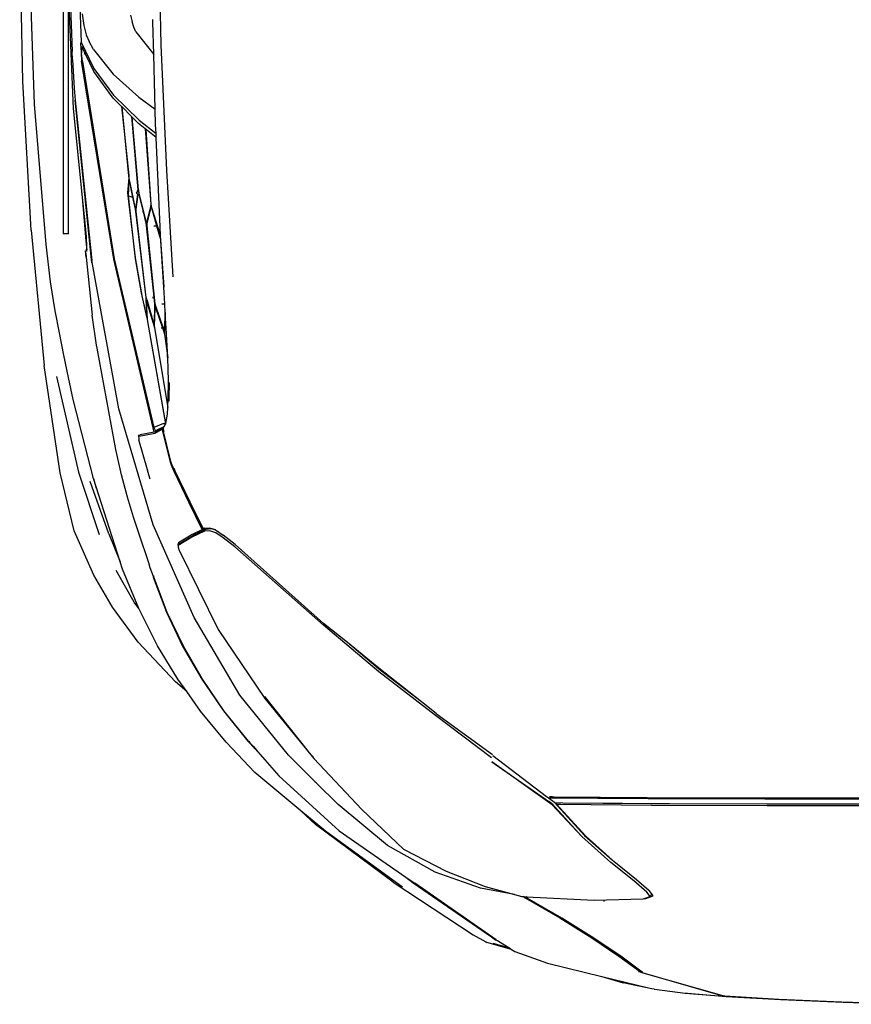
# Model space of a CAD drawing. Units: inches. Extents: x 22042254 to 25404563, y 17568978 to 17626777.
# Tile 1 of 45: x 22042254.0718 to 22042254.4976, y 17568977.6618 to 17568978.1657. Entities that reach past the tile are written whole.
import ezdxf

# ---------------------------------------------------------------- set-up
doc = ezdxf.new("R2010")
doc.units = ezdxf.units.IN
doc.header["$MEASUREMENT"] = 0
doc.layers.add('A-SITE-VEHI', color=8, linetype='Continuous', lineweight=18)
doc.layers.add('Edges', color=250, linetype='Continuous')

# ---------------------------------------------------------------- blocks, each defined once
blk = doc.blocks.new('Nissan Qashqai pl')
at = {"layer": 'Edges'}
for p, q in [((8.01597, 12.81888), (7.96577, 12.81715)), ((7.96683, 12.81735), (8.01677, 12.81906)), ((7.86763, 12.81233), (7.79979, 12.79282)), ((7.80119, 12.79291), (7.86805, 12.81214)), ((7.83626, 12.80972), (7.86763, 12.81233)), ((7.83812, 12.80996), (7.86997, 12.81262)), ((7.86763, 12.81233), (7.86805, 12.81214)), ((7.86903, 12.81242), (7.86805, 12.81214)), ((7.91369, 12.81497), (7.86903, 12.81242)), ((7.86997, 12.81262), (7.91514, 12.8152)), ((7.96577, 12.81715), (7.91369, 12.81497)), ((7.91514, 12.8152), (7.96683, 12.81735)), ((7.7673, 12.79611), (7.80585, 12.80552)), ((7.80866, 12.80621), (7.78484, 12.80117)), ((7.79357, 12.80288), (7.79772, 12.80375)), ((7.81062, 12.80645), (7.80866, 12.80621)), ((7.81062, 12.80645), (7.81073, 12.80648)), ((7.81073, 12.80648), (7.83626, 12.80972)), ((7.83626, 12.80972), (7.83812, 12.80996)), ((7.72226, 12.78511), (7.7673, 12.79611)), ((7.7673, 12.79611), (7.78484, 12.80117)), ((7.78354, 12.80068), (7.78351, 12.80067)), ((7.78647, 12.80131), (7.78656, 12.80134)), ((7.78138, 12.77913), (7.79909, 12.7923)), ((7.79842, 12.79085), (7.78285, 12.7793)), ((7.79759, 12.79204), (7.79909, 12.7923)), ((7.80074, 12.79258), (7.79842, 12.79085)), ((7.79909, 12.7923), (7.79979, 12.79282)), ((7.79952, 12.79237), (7.80074, 12.79258)), ((7.80119, 12.79291), (7.80074, 12.79258)), ((7.69527, 12.77535), (7.72226, 12.78511)), ((7.75906, 12.76414), (7.78138, 12.77913)), ((7.78285, 12.7793), (7.76061, 12.76436)), ((7.6926, 12.77369), (7.67207, 12.76794)), ((7.69111, 12.77277), (7.67743, 12.76878)), ((7.68089, 12.76644), (7.69111, 12.77277)), ((7.69111, 12.77277), (7.6926, 12.77369)), ((7.6926, 12.77369), (7.69527, 12.77535)), ((7.59458, 12.71797), (7.66077, 12.76166)), ((7.61132, 12.71859), (7.67585, 12.76329)), ((7.67993, 12.76585), (7.61247, 12.71901)), ((7.66077, 12.76166), (7.67122, 12.76746)), ((7.67122, 12.76746), (7.67207, 12.76794)), ((7.67585, 12.76329), (7.67933, 12.76572)), ((7.67933, 12.76572), (7.68018, 12.766)), ((7.67993, 12.76585), (7.68018, 12.766)), ((7.68018, 12.766), (7.68089, 12.76644)), ((7.73247, 12.74757), (7.75906, 12.76414)), ((7.76061, 12.76436), (7.73411, 12.74784)), ((7.70382, 12.731), (7.73247, 12.74757)), ((7.73411, 12.74784), (7.70559, 12.73137)), ((7.69488, 12.72832), (7.70101, 12.73001)), ((7.70101, 12.73001), (7.70235, 12.73008)), ((7.70235, 12.73008), (7.70382, 12.731)), ((7.70235, 12.73008), (7.70343, 12.73013)), ((7.70559, 12.73137), (7.70343, 12.73013)), ((7.70343, 12.73013), (7.70481, 12.7302)), ((7.70481, 12.7302), (7.76082, 12.73292)), ((7.70579, 12.73076), (7.70481, 12.7302)), ((7.76082, 12.73292), (7.80143, 12.73178)), ((7.76878, 12.73282), (7.76885, 12.73399)), ((7.80143, 12.73178), (7.80216, 12.73156)), ((7.80216, 12.73156), (7.80372, 12.73151)), ((7.80216, 12.73156), (7.80721, 12.73004)), ((7.80372, 12.73151), (7.80956, 12.72941)), ((7.80721, 12.73004), (7.80447, 12.72626)), ((7.80956, 12.72941), (7.80665, 12.72539)), ((7.80721, 12.73004), (7.80867, 12.72831)), ((7.60245, 12.72211), (7.53868, 12.67594)), ((7.66697, 12.723), (7.62951, 12.70974)), ((7.63858, 12.70891), (7.67084, 12.72167)), ((7.69488, 12.72832), (7.66697, 12.723)), ((7.67084, 12.72167), (7.69488, 12.72832)), ((7.80447, 12.72626), (7.79381, 12.71706)), ((7.80619, 12.725), (7.79586, 12.71608)), ((7.80619, 12.725), (7.80867, 12.72831)), ((7.80665, 12.72539), (7.80619, 12.725)), ((7.59458, 12.71797), (7.53043, 12.67044)), ((7.55011, 12.67573), (7.60515, 12.71393)), ((7.60515, 12.71393), (7.61132, 12.71859)), ((7.60515, 12.71393), (7.61111, 12.71807)), ((7.61183, 12.71862), (7.61111, 12.71807)), ((7.61247, 12.71901), (7.61183, 12.71862)), ((7.79381, 12.71706), (7.77477, 12.70185)), ((7.79586, 12.71608), (7.77724, 12.70105)), ((7.62951, 12.70974), (7.58999, 12.68766)), ((7.60319, 12.69082), (7.63858, 12.70891)), ((7.77477, 12.70185), (7.75074, 12.68033)), ((7.75301, 12.67941), (7.77596, 12.69989)), ((7.77596, 12.69989), (7.75388, 12.67998)), ((7.77724, 12.70105), (7.77596, 12.69989)), ((7.56866, 12.65792), (7.60319, 12.69082)), ((7.58999, 12.68766), (7.5492, 12.654)), ((7.72614, 12.65431), (7.75074, 12.68033)), ((7.75074, 12.68033), (7.72856, 12.65607)), ((7.55011, 12.67573), (7.50008, 12.63025)), ((7.53868, 12.67594), (7.5184, 12.65911)), ((7.75301, 12.67941), (7.72807, 12.65235)), ((7.75388, 12.67998), (7.73238, 12.65652)), ((7.5184, 12.65911), (7.53043, 12.67044)), ((7.5184, 12.65911), (7.48015, 12.62736)), ((7.52891, 12.61585), (7.56866, 12.65792)), ((7.72856, 12.65607), (7.72667, 12.65393)), ((7.73238, 12.65652), (7.72986, 12.65372)), ((7.5492, 12.654), (7.53101, 12.63591)), ((7.72614, 12.65431), (7.67617, 12.61859)), ((7.67617, 12.61859), (7.72327, 12.65136)), ((7.7215, 12.64734), (7.72214, 12.64782)), ((7.72318, 12.64862), (7.72214, 12.64782)), ((7.72807, 12.65235), (7.72318, 12.64862)), ((7.72455, 12.64863), (7.72318, 12.64862)), ((7.72667, 12.65393), (7.72327, 12.65136)), ((7.72606, 12.64765), (7.72382, 12.64759)), ((7.72942, 12.64868), (7.72455, 12.64863)), ((7.72785, 12.6477), (7.72606, 12.64765)), ((7.80482, 12.64828), (7.72785, 12.6477)), ((7.72986, 12.65372), (7.72807, 12.65235)), ((7.72807, 12.65235), (7.73491, 12.65241)), ((7.73098, 12.64869), (7.72942, 12.64868)), ((7.72986, 12.65372), (7.73345, 12.65375)), ((7.76399, 12.64888), (7.73098, 12.64869)), ((7.73345, 12.65375), (7.80829, 12.65437)), ((7.73491, 12.65241), (7.76799, 12.65269)), ((7.76622, 12.64889), (7.76399, 12.64888)), ((7.78115, 12.64897), (7.76622, 12.64889)), ((7.76799, 12.65269), (7.76925, 12.6527)), ((7.76925, 12.6527), (7.78439, 12.65283)), ((7.78224, 12.64898), (7.78115, 12.64897)), ((7.80566, 12.64911), (7.78224, 12.64898)), ((7.78439, 12.65283), (7.80777, 12.65303)), ((7.90142, 12.64867), (7.80482, 12.64828)), ((7.82329, 12.64918), (7.80566, 12.64911)), ((7.80777, 12.65303), (7.82329, 12.65309)), ((7.80829, 12.65437), (7.90396, 12.65472)), ((7.82329, 12.65309), (7.90357, 12.65342)), ((7.90204, 12.64948), (7.82329, 12.64918)), ((8.02732, 12.64849), (7.90142, 12.64867)), ((8.02749, 12.64934), (7.90204, 12.64948)), ((7.90357, 12.65342), (8.0275, 12.6533)), ((7.90396, 12.65472), (8.02759, 12.65454)), ((7.67714, 12.61347), (7.7215, 12.64734)), ((7.53101, 12.63591), (7.50805, 12.61306)), ((7.53101, 12.63591), (7.53009, 12.6353)), ((7.48015, 12.62736), (7.45654, 12.6023)), ((7.48274, 12.61035), (7.50008, 12.63025)), ((7.48836, 12.56635), (7.52891, 12.61585)), ((7.67598, 12.61523), (7.6296, 12.58026)), ((7.50805, 12.61306), (7.46788, 12.56344)), ((7.47438, 12.60148), (7.48041, 12.60787)), ((7.48041, 12.60787), (7.47799, 12.6049)), ((7.47901, 12.60607), (7.4815, 12.60892)), ((7.47901, 12.60607), (7.48009, 12.6074)), ((7.48009, 12.6074), (7.48041, 12.60787)), ((7.48041, 12.60787), (7.48043, 12.60789)), ((7.48043, 12.60789), (7.48069, 12.60817)), ((7.48069, 12.60817), (7.48214, 12.60971)), ((7.4815, 12.60892), (7.48214, 12.60971)), ((7.48214, 12.60971), (7.48274, 12.61035)), ((7.48817, 12.5645), (7.52431, 12.61007)), ((7.52431, 12.61007), (7.52857, 12.61458)), ((7.67691, 12.61295), (7.63059, 12.57913)), ((7.45654, 12.6023), (7.4354, 12.57664)), ((7.45423, 12.57648), (7.47438, 12.60148)), ((7.47504, 12.60161), (7.45491, 12.57668)), ((7.47616, 12.6028), (7.47504, 12.60161)), ((7.47515, 12.60164), (7.47616, 12.6028)), ((7.47616, 12.6028), (7.47799, 12.6049)), ((7.47799, 12.6049), (7.47901, 12.60607)), ((7.4354, 12.57664), (7.42386, 12.56045)), ((7.43626, 12.55019), (7.45423, 12.57648)), ((7.45491, 12.57668), (7.4369, 12.55039)), ((7.6296, 12.58026), (7.58274, 12.54411)), ((7.63007, 12.57872), (7.61803, 12.56913)), ((7.63059, 12.57913), (7.63007, 12.57872)), ((7.44978, 12.50928), (7.48836, 12.56635)), ((7.61803, 12.56913), (7.58288, 12.54113)), ((7.61803, 12.56913), (7.58398, 12.54289)), ((7.42386, 12.56045), (7.41469, 12.55237)), ((7.42386, 12.56045), (7.41661, 12.55027)), ((7.46788, 12.56344), (7.43015, 12.49926)), ((7.41469, 12.55237), (7.38367, 12.51969)), ((7.41661, 12.55027), (7.39973, 12.5227)), ((7.42053, 12.52292), (7.43626, 12.55019)), ((7.4369, 12.55039), (7.42115, 12.52316)), ((7.58274, 12.54411), (7.53689, 12.50568)), ((7.58398, 12.54289), (7.55683, 12.52012)), ((7.58288, 12.54113), (7.55683, 12.52012)), ((7.38367, 12.51969), (7.36237, 12.49067)), ((7.39973, 12.5227), (7.38446, 12.49246)), ((7.40715, 12.49483), (7.42053, 12.52292)), ((7.42115, 12.52316), (7.40781, 12.49514)), ((7.55683, 12.52012), (7.53708, 12.50419)), ((7.41723, 12.44309), (7.44978, 12.50928)), ((7.53689, 12.50568), (7.46355, 12.44079)), ((7.46382, 12.43903), (7.53708, 12.50419)), ((7.39621, 12.46602), (7.40715, 12.49483)), ((7.43015, 12.49926), (7.39627, 12.4227)), ((7.40781, 12.49514), (7.39687, 12.46646)), ((7.36237, 12.49067), (7.34698, 12.4644)), ((7.38053, 12.48658), (7.36552, 12.46044)), ((7.38426, 12.49197), (7.37074, 12.45925)), ((7.38426, 12.49197), (7.38053, 12.48658)), ((7.38446, 12.49246), (7.38426, 12.49197)), ((7.34698, 12.4644), (7.3309, 12.42757)), ((7.39513, 12.46199), (7.39379, 12.45826)), ((7.39648, 12.46548), (7.39513, 12.46199)), ((7.39648, 12.46548), (7.39621, 12.46602)), ((7.39687, 12.46646), (7.39648, 12.46548)), ((7.39676, 12.46492), (7.39668, 12.46506)), ((7.3688, 12.45323), (7.34671, 12.38455)), ((7.35959, 12.43024), (7.3688, 12.45323)), ((7.37074, 12.45925), (7.3688, 12.45323)), ((7.39247, 12.45422), (7.38454, 12.43058)), ((7.39379, 12.45826), (7.39247, 12.45422)), ((7.41665, 12.43928), (7.41687, 12.44057)), ((7.41665, 12.43928), (7.41716, 12.43948)), ((7.41697, 12.43768), (7.41665, 12.43928)), ((7.41686, 12.44121), (7.41723, 12.44309)), ((7.41687, 12.44057), (7.41686, 12.44121)), ((7.41687, 12.44057), (7.41717, 12.44232)), ((7.41689, 12.43978), (7.41687, 12.44057)), ((7.42821, 12.43284), (7.41689, 12.43978)), ((7.41716, 12.43948), (7.41689, 12.43978)), ((7.42833, 12.4307), (7.41697, 12.43768)), ((7.4183, 12.4382), (7.41716, 12.43948)), ((7.41717, 12.44232), (7.41744, 12.44287)), ((7.41747, 12.44292), (7.41744, 12.44287)), ((7.4183, 12.4382), (7.42961, 12.43124)), ((7.46355, 12.44079), (7.4541, 12.43335)), ((7.46382, 12.43903), (7.45415, 12.43132)), ((7.33449, 12.37926), (7.3514, 12.43082)), ((7.35959, 12.43024), (7.34401, 12.38695)), ((7.38454, 12.43058), (7.37986, 12.41639)), ((7.43873, 12.42797), (7.42821, 12.43284)), ((7.43587, 12.42718), (7.42833, 12.4307)), ((7.43832, 12.42716), (7.42961, 12.43124)), ((7.44309, 12.42761), (7.43873, 12.42797)), ((7.44789, 12.42929), (7.44309, 12.42761)), ((7.44771, 12.42699), (7.45415, 12.43132)), ((7.4541, 12.43335), (7.44789, 12.42929)), ((7.3309, 12.42757), (7.31925, 12.37966)), ((7.39627, 12.4227), (7.36761, 12.32692)), ((7.42553, 12.40435), (7.43673, 12.42678)), ((7.43648, 12.4235), (7.42672, 12.4041)), ((7.43673, 12.42678), (7.43587, 12.42718)), ((7.43651, 12.42353), (7.43648, 12.4235)), ((7.43782, 12.42614), (7.43651, 12.42353)), ((7.43673, 12.42678), (7.43832, 12.42716)), ((7.43787, 12.42625), (7.43782, 12.42614)), ((7.43787, 12.42625), (7.43832, 12.42716)), ((7.43787, 12.42625), (7.4389, 12.42689)), ((7.43844, 12.42599), (7.43787, 12.42625)), ((7.43844, 12.42599), (7.43799, 12.42508)), ((7.43832, 12.42716), (7.4389, 12.42689)), ((7.4389, 12.42689), (7.43844, 12.42599)), ((7.43873, 12.42586), (7.43844, 12.42599)), ((7.44298, 12.42535), (7.43873, 12.42586)), ((7.44004, 12.42635), (7.4389, 12.42689)), ((7.44004, 12.42635), (7.44418, 12.42585)), ((7.44771, 12.42699), (7.44298, 12.42535)), ((7.44418, 12.42585), (7.44771, 12.42699)), ((7.37986, 12.41639), (7.375, 12.39997)), ((7.41315, 12.3783), (7.42553, 12.40435)), ((7.42672, 12.4041), (7.41393, 12.37779)), ((7.375, 12.39997), (7.36995, 12.3813)), ((7.34671, 12.38455), (7.34891, 12.39245)), ((7.31925, 12.37966), (7.3059, 12.29098)), ((7.31612, 12.30008), (7.33449, 12.37926)), ((7.34671, 12.38455), (7.32996, 12.31924)), ((7.36995, 12.3813), (7.36534, 12.36039)), ((7.39248, 12.38132), (7.39136, 12.37745)), ((7.39374, 12.38511), (7.39248, 12.38132)), ((7.39133, 12.37737), (7.38437, 12.35258)), ((7.39133, 12.37737), (7.39136, 12.37745)), ((7.40326, 12.3435), (7.41007, 12.37083)), ((7.41007, 12.37083), (7.41147, 12.37465)), ((7.41219, 12.37416), (7.41077, 12.37034)), ((7.41147, 12.37465), (7.41315, 12.3783)), ((7.41393, 12.37779), (7.41219, 12.37416)), ((7.41334, 12.37586), (7.41416, 12.37763)), ((7.41077, 12.37034), (7.40418, 12.34346)), ((7.36534, 12.36039), (7.3497, 12.27675)), ((7.38412, 12.34854), (7.38437, 12.35258)), ((7.38458, 12.34953), (7.38412, 12.34854)), ((7.38412, 12.34854), (7.38529, 12.34833)), ((7.38458, 12.34953), (7.39764, 12.34702)), ((7.39705, 12.34608), (7.38529, 12.34833)), ((7.39764, 12.34702), (7.40264, 12.34394)), ((7.39705, 12.34608), (7.36347, 12.20326)), ((7.36397, 12.20287), (7.39678, 12.34241)), ((7.39156, 12.25473), (7.40622, 12.33886)), ((7.40648, 12.33918), (7.39169, 12.25467)), ((7.39678, 12.34241), (7.39804, 12.34491)), ((7.40464, 12.33886), (7.39678, 12.34241)), ((7.39833, 12.34584), (7.39705, 12.34608)), ((7.39804, 12.34491), (7.39989, 12.34404)), ((7.39804, 12.34491), (7.4012, 12.34407)), ((7.4012, 12.34407), (7.39833, 12.34584)), ((7.39989, 12.34404), (7.40511, 12.34151)), ((7.39989, 12.34404), (7.40478, 12.34174)), ((7.40335, 12.34275), (7.4012, 12.34407)), ((7.4012, 12.34407), (7.40147, 12.344)), ((7.40147, 12.344), (7.40276, 12.34374)), ((7.40264, 12.34394), (7.40326, 12.3435)), ((7.40326, 12.3435), (7.40417, 12.34217)), ((7.40417, 12.34217), (7.40335, 12.34275)), ((7.40418, 12.34346), (7.40405, 12.34294)), ((7.40405, 12.34294), (7.40431, 12.34276)), ((7.40405, 12.34294), (7.40425, 12.34252)), ((7.40411, 12.34347), (7.40418, 12.34346)), ((7.40417, 12.34217), (7.40425, 12.34252)), ((7.40443, 12.34217), (7.40417, 12.34217)), ((7.40418, 12.34346), (7.40447, 12.3434)), ((7.40425, 12.34252), (7.40431, 12.34276)), ((7.40425, 12.34252), (7.40443, 12.34217)), ((7.40431, 12.34276), (7.40447, 12.3434)), ((7.40431, 12.34276), (7.40461, 12.34255)), ((7.40443, 12.34217), (7.40456, 12.34189)), ((7.40463, 12.34217), (7.40443, 12.34217)), ((7.40447, 12.3434), (7.40502, 12.34562)), ((7.40447, 12.3434), (7.4048, 12.34334)), ((7.40463, 12.34217), (7.40456, 12.34189)), ((7.40456, 12.34189), (7.40497, 12.34189)), ((7.40478, 12.34174), (7.40456, 12.34189)), ((7.40461, 12.34255), (7.40469, 12.3424)), ((7.40469, 12.3424), (7.40463, 12.34217)), ((7.40482, 12.34217), (7.40463, 12.34217)), ((7.40464, 12.33886), (7.40622, 12.33886)), ((7.40469, 12.3424), (7.40482, 12.34217)), ((7.40478, 12.34174), (7.40515, 12.34156)), ((7.40511, 12.34151), (7.40478, 12.34174)), ((7.40482, 12.34217), (7.40497, 12.34189)), ((7.40497, 12.34189), (7.40515, 12.34156)), ((7.40511, 12.34151), (7.40521, 12.34146)), ((7.40515, 12.34156), (7.40521, 12.34146)), ((7.40521, 12.34146), (7.40632, 12.33946)), ((7.40622, 12.33886), (7.40632, 12.33946)), ((7.40632, 12.33946), (7.40648, 12.33918)), ((7.40648, 12.33918), (7.4066, 12.33895)), ((7.4066, 12.33895), (7.40795, 12.33127)), ((7.40795, 12.33127), (7.40828, 12.32581)), ((7.36761, 12.32692), (7.34554, 12.2042)), ((7.39714, 12.25992), (7.40828, 12.32581)), ((7.40836, 12.3244), (7.39747, 12.25989)), ((7.40828, 12.32581), (7.40836, 12.3244)), ((7.40836, 12.3244), (7.40865, 12.31952)), ((7.32996, 12.31924), (7.3261, 12.30088)), ((7.40865, 12.31952), (7.40871, 12.30369)), ((7.40921, 12.31837), (7.40908, 12.32063)), ((7.40923, 12.30498), (7.40921, 12.31837)), ((7.3261, 12.30088), (7.32232, 12.28252)), ((7.40871, 12.30369), (7.40814, 12.28481)), ((7.29513, 12.17908), (7.3059, 12.29098)), ((7.32232, 12.28252), (7.3186, 12.26414)), ((7.40539, 12.2651), (7.40814, 12.28481)), ((7.40811, 12.28378), (7.40791, 12.2798)), ((7.40814, 12.28481), (7.40811, 12.28378)), ((7.34938, 12.27412), (7.34574, 12.2495)), ((7.34978, 12.2768), (7.34938, 12.27412)), ((7.3497, 12.27675), (7.34938, 12.27412)), ((7.40791, 12.2798), (7.40588, 12.26512)), ((7.40791, 12.2798), (7.40687, 12.2598)), ((7.40488, 12.26309), (7.40539, 12.2651)), ((7.40588, 12.26512), (7.40585, 12.26319)), ((7.3186, 12.26414), (7.31494, 12.24575)), ((7.39095, 12.23871), (7.39668, 12.25792)), ((7.39691, 12.257), (7.39654, 12.25604)), ((7.39668, 12.25792), (7.39714, 12.25992)), ((7.39684, 12.25593), (7.39691, 12.257)), ((7.39747, 12.25989), (7.39733, 12.25795)), ((7.39733, 12.25795), (7.39774, 12.24387)), ((7.40485, 12.26124), (7.39823, 12.24191)), ((7.39827, 12.24398), (7.40376, 12.25987)), ((7.40279, 12.25987), (7.40376, 12.25987)), ((7.40376, 12.25987), (7.40488, 12.26309)), ((7.40532, 12.26222), (7.40485, 12.26124)), ((7.40532, 12.26117), (7.40532, 12.26222)), ((7.40611, 12.24728), (7.40532, 12.26117)), ((7.40592, 12.26183), (7.40555, 12.26207)), ((7.40585, 12.26319), (7.40592, 12.26183)), ((7.40592, 12.26183), (7.40642, 12.25231)), ((7.40687, 12.2598), (7.40642, 12.25231)), ((7.3407, 12.2016), (7.34574, 12.2495)), ((7.39089, 12.25084), (7.38644, 12.23105)), ((7.3869, 12.23473), (7.39116, 12.25274)), ((7.39012, 12.23681), (7.39099, 12.25068)), ((7.39141, 12.25272), (7.39058, 12.23864)), ((7.3908, 12.23661), (7.39654, 12.25604)), ((7.39114, 12.25178), (7.39089, 12.25084)), ((7.39099, 12.25068), (7.39114, 12.25178)), ((7.39121, 12.25173), (7.39114, 12.25178)), ((7.39116, 12.25274), (7.39156, 12.25473)), ((7.39169, 12.25467), (7.39141, 12.25272)), ((7.39722, 12.24205), (7.39684, 12.25593)), ((7.40642, 12.25231), (7.40611, 12.24728)), ((7.31494, 12.24575), (7.31133, 12.22174)), ((7.39715, 12.24), (7.39722, 12.24205)), ((7.39823, 12.24191), (7.39768, 12.23999)), ((7.39774, 12.24387), (7.39795, 12.24289)), ((7.39795, 12.24289), (7.39827, 12.24398)), ((7.40611, 12.2472), (7.40567, 12.23998)), ((7.40611, 12.2472), (7.40611, 12.24728)), ((7.38128, 12.20212), (7.3869, 12.23473)), ((7.38152, 12.16381), (7.38995, 12.23475)), ((7.39032, 12.23471), (7.38195, 12.16385)), ((7.38995, 12.23475), (7.39012, 12.23681)), ((7.3908, 12.23661), (7.39032, 12.23471)), ((7.39046, 12.17543), (7.3966, 12.23466)), ((7.39058, 12.23864), (7.39067, 12.23763)), ((7.39067, 12.23763), (7.39095, 12.23871)), ((7.39768, 12.23999), (7.39107, 12.17551)), ((7.39566, 12.23466), (7.3966, 12.23466)), ((7.3957, 12.2348), (7.39661, 12.2348)), ((7.3966, 12.23466), (7.39661, 12.2348)), ((7.39661, 12.2348), (7.39715, 12.24)), ((7.40319, 12.23998), (7.40567, 12.23998)), ((7.40567, 12.23998), (7.40484, 12.22617)), ((7.38644, 12.23105), (7.38154, 12.2029)), ((7.40216, 12.18704), (7.40484, 12.22617)), ((7.40484, 12.22617), (7.40226, 12.1836)), ((7.31133, 12.22174), (7.30777, 12.19099)), ((7.40723, 12.12993), (7.41241, 12.21762)), ((7.34554, 12.20616), (7.33168, 12.07174)), ((7.33168, 12.07174), (7.34554, 12.2042)), ((7.3407, 12.2016), (7.34004, 12.19617)), ((7.34033, 12.19813), (7.3407, 12.2016)), ((7.36347, 12.20326), (7.34048, 12.06162)), ((7.34263, 12.07068), (7.36397, 12.20287)), ((7.37498, 12.14844), (7.38128, 12.20212)), ((7.38154, 12.2029), (7.37562, 12.1509)), ((7.34004, 12.19617), (7.34009, 12.19616)), ((7.34009, 12.19616), (7.34097, 12.1962)), ((7.34131, 12.19329), (7.34072, 12.18787)), ((7.34097, 12.1962), (7.341, 12.1962)), ((7.34097, 12.1962), (7.34131, 12.19329)), ((7.34133, 12.19308), (7.34097, 12.18475)), ((7.341, 12.1962), (7.34144, 12.1962)), ((7.34145, 12.19617), (7.341, 12.1962)), ((7.34154, 12.19537), (7.34131, 12.19329)), ((7.34131, 12.19329), (7.34133, 12.19308)), ((7.30777, 12.19099), (7.29801, 12.07497)), ((7.34072, 12.18787), (7.33778, 12.15206)), ((7.34097, 12.18475), (7.33996, 12.17312)), ((7.39898, 12.17558), (7.4017, 12.185)), ((7.4017, 12.185), (7.40216, 12.18704)), ((7.40226, 12.1836), (7.40182, 12.17639)), ((7.40226, 12.1836), (7.40207, 12.18329)), ((7.29513, 12.17908), (7.28835, 12.05625)), ((7.32607, 12.18208), (7.32157, 12.18208)), ((7.32157, 11.66208), (7.32157, 12.18208)), ((7.32607, 12.18208), (7.32607, 11.97794)), ((7.39008, 12.17342), (7.39046, 12.17543)), ((7.39107, 12.17551), (7.39127, 12.17366)), ((7.39494, 12.16159), (7.39898, 12.17558)), ((7.40207, 12.18329), (7.39509, 12.16063)), ((7.39666, 12.17558), (7.39898, 12.17558)), ((7.40182, 12.17639), (7.39862, 12.10249)), ((7.33996, 12.17312), (7.33778, 12.15206)), ((7.39028, 12.17165), (7.38438, 12.14787)), ((7.38773, 12.16389), (7.39008, 12.17342)), ((7.39074, 12.17265), (7.39028, 12.17165)), ((7.39087, 12.17164), (7.39074, 12.17265)), ((7.39387, 12.15956), (7.39087, 12.17164)), ((7.39127, 12.17366), (7.39425, 12.16142)), ((7.38127, 12.15992), (7.37634, 12.13606)), ((7.37916, 12.15176), (7.38118, 12.1619)), ((7.38118, 12.1619), (7.38152, 12.16381)), ((7.38146, 12.16096), (7.38127, 12.15992)), ((7.3817, 12.16004), (7.38146, 12.16096)), ((7.38322, 12.1493), (7.3817, 12.16004)), ((7.38195, 12.16385), (7.38202, 12.1619)), ((7.38202, 12.1619), (7.38379, 12.14973)), ((7.38426, 12.14979), (7.38773, 12.16389)), ((7.38773, 12.16389), (7.38737, 12.16389)), ((7.39414, 12.15763), (7.39387, 12.15956)), ((7.39425, 12.16142), (7.39471, 12.16054)), ((7.39509, 12.16063), (7.39449, 12.15768)), ((7.39471, 12.16054), (7.39494, 12.16159)), ((7.33778, 12.15206), (7.33017, 12.07853)), ((7.37562, 12.1509), (7.37916, 12.15176)), ((7.37642, 12.13802), (7.37916, 12.15176)), ((7.38964, 12.09538), (7.39414, 12.15763)), ((7.39449, 12.15768), (7.39027, 12.09589)), ((7.37596, 12.13603), (7.37498, 12.14844)), ((7.37562, 12.1509), (7.37623, 12.13799)), ((7.37826, 12.0852), (7.38357, 12.14586)), ((7.38403, 12.14592), (7.37876, 12.0857)), ((7.38322, 12.1493), (7.38243, 12.1487)), ((7.38243, 12.1487), (7.38324, 12.14918)), ((7.38357, 12.14586), (7.38243, 12.1487)), ((7.38243, 12.1487), (7.3835, 12.14683)), ((7.38379, 12.14973), (7.38322, 12.1493)), ((7.38324, 12.14918), (7.38322, 12.1493)), ((7.38324, 12.14918), (7.38374, 12.14948)), ((7.38357, 12.14586), (7.3835, 12.14683)), ((7.3835, 12.14683), (7.38403, 12.14592)), ((7.38374, 12.14948), (7.38426, 12.14979)), ((7.38374, 12.14948), (7.38379, 12.14973)), ((7.38403, 12.14592), (7.38424, 12.1495)), ((7.38438, 12.14787), (7.38403, 12.14592)), ((7.38424, 12.1495), (7.38426, 12.14979)), ((7.38427, 12.14952), (7.38424, 12.1495)), ((7.37589, 12.1341), (7.37596, 12.13603)), ((7.37634, 12.13606), (7.37608, 12.13413)), ((7.37623, 12.13799), (7.37624, 12.13703)), ((7.37624, 12.13703), (7.37642, 12.13802)), ((7.37638, 12.13711), (7.37624, 12.13703)), ((7.37008, 12.07708), (7.37589, 12.1341)), ((7.37608, 12.13413), (7.37036, 12.07735)), ((7.40245, 12.02601), (7.40723, 12.12993)), ((7.39862, 12.10249), (7.39027, 12.09589)), ((7.39862, 12.10249), (7.39848, 12.09934)), ((7.38964, 12.09538), (7.38409, 12.09099)), ((7.38449, 12.08832), (7.39848, 12.09934)), ((7.39027, 12.09589), (7.38964, 12.09538)), ((7.39848, 12.09934), (7.39816, 12.09205)), ((7.36331, 12.06744), (7.38449, 12.08832)), ((7.38409, 12.09099), (7.37876, 12.0857)), ((7.39816, 12.09205), (7.39782, 12.07909)), ((7.33017, 12.07853), (7.32607, 11.97794)), ((7.37826, 12.0852), (7.37036, 12.07735)), ((7.37876, 12.0857), (7.37826, 12.0852)), ((7.38423, 12.06929), (7.39782, 12.07909)), ((7.39782, 12.07909), (7.3966, 12.03384)), ((7.29801, 12.07497), (7.29279, 11.92208)), ((7.33087, 12.06192), (7.33168, 12.07174)), ((7.34104, 12.06045), (7.34263, 12.07068)), ((7.36309, 12.07013), (7.34693, 12.0481)), ((7.37008, 12.07708), (7.36309, 12.07013)), ((7.37036, 12.07735), (7.37008, 12.07708)), ((7.32941, 12.03847), (7.33087, 12.06192)), ((7.34048, 12.06162), (7.33691, 12.03944)), ((7.34711, 12.04544), (7.36331, 12.06744)), ((7.36303, 12.05012), (7.38423, 12.06929)), ((7.28835, 12.05625), (7.28572, 11.92208)), ((7.33767, 12.03978), (7.34104, 12.06045)), ((7.33653, 12.02372), (7.34711, 12.04544)), ((7.34693, 12.0481), (7.3402, 12.0337)), ((7.34679, 12.02992), (7.36303, 12.05012)), ((7.32941, 12.03847), (7.32911, 12.03155)), ((7.33645, 12.03215), (7.33691, 12.03944)), ((7.33767, 12.03978), (7.33691, 12.03284)), ((7.32507, 11.92208), (7.32911, 12.03155)), ((7.33615, 12.02477), (7.33645, 12.03215)), ((7.33686, 12.0287), (7.33691, 12.03284)), ((7.33805, 12.02908), (7.33686, 12.0287)), ((7.33805, 12.02908), (7.33737, 12.02763)), ((7.3402, 12.0337), (7.33805, 12.02908)), ((7.33873, 12.03324), (7.3402, 12.0337)), ((7.34679, 12.02992), (7.34316, 12.02313)), ((7.38184, 12.0151), (7.3966, 12.03384)), ((7.3966, 12.03384), (7.39589, 12.00706)), ((7.33294, 11.92208), (7.33653, 12.02372)), ((7.33615, 12.02477), (7.33659, 12.02464)), ((7.33653, 12.02372), (7.33615, 12.02477)), ((7.33737, 12.02763), (7.33686, 12.0287)), ((7.3407, 12.01758), (7.34316, 12.02313)), ((7.40018, 11.92208), (7.40245, 12.02601)), ((7.33865, 12.00996), (7.3407, 12.01758)), ((7.38184, 12.0151), (7.38014, 12.01146)), ((7.33733, 12.00038), (7.33865, 12.00996)), ((7.37751, 12.0015), (7.37864, 12.00699)), ((7.38014, 12.01146), (7.37864, 12.00699)), ((7.39589, 12.00706), (7.39588, 12.00508))]:
    blk.add_line(p, q, dxfattribs=at)
blk = doc.blocks.new('CAR')
blk.add_blockref('Nissan Qashqai pl', (-9.74328, -11.91512))

msp = doc.modelspace()

# ---------------------------------------------------------------- block references
at = {"layer": 'A-SITE-VEHI', "xscale": -0.6191396643141144, "yscale": 0.6191396643141144, "zscale": 0.6191396643141144, "rotation": 180}
msp.add_blockref('CAR', (22042255.59333, 17568978.22147), dxfattribs=at)

doc.saveas('drawing.dxf')
